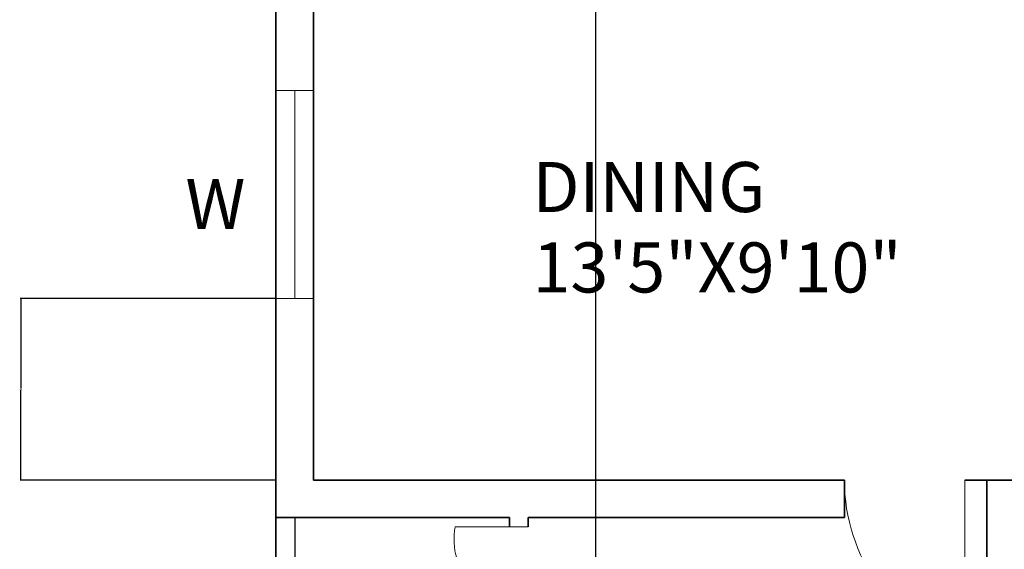
# Model space of a CAD drawing. Units: feet. Extents: x 5816 to 6644, y 25475 to 26788.
# Tile 5 of 23: x 5816 to 6052, y 26246 to 26373. Entities that reach past the tile are written whole.
import ezdxf

# ---------------------------------------------------------------- set-up
doc = ezdxf.new("R2010")
doc.units = ezdxf.units.FT
for name, color, linetype, lineweight in [('A-ANNO-DIMS', 2, 'Continuous', 13), ('A-ANNO-TEXT', 7, 'Continuous', 18), ('A-AREA-IDEN', 7, 'Continuous', 18), ('A-DOOR', 3, 'Continuous', 18), ('A-FLOR-RAIL', 8, 'Continuous', 25), ('A-GLAZ', 4, 'Continuous', 18), ('A-WALL', 7, 'Continuous', 35)]:
    doc.layers.add(name, color=color, linetype=linetype, lineweight=lineweight)
doc.styles.get("Standard").update_dxf_attribs({"font": 'arial.ttf'})
doc.dimstyles.get("Standard").update_dxf_attribs({"dimtxt": 0.18, "dimasz": 0.18, "dimexe": 0.18, "dimexo": 0.0625, "dimgap": 0.09, "dimtad": 0, "dimtih": 1, "dimtoh": 1, "dimdec": 4, "dimzin": 0, "dimdsep": 46, "dimtxsty": 'Standard', "dimcen": 0.09, "dimadec": 0, "dimazin": 0, "dimtfac": 1, "dimtdec": 4, "dimtofl": 0, "dimtmove": 0, "dimatfit": 3, "dimfxl": 1, "dimtolj": 1, "dimtzin": 0, "dimarcsym": 0})

# ---------------------------------------------------------------- blocks, each defined once
blk = doc.blocks.new('DOOR-KITCHEN')
blk.add_line((0, -40.87), (0, 0))
blk.add_arc((14.45, 0), 43.35, 180, 250.5286)
blk = doc.blocks.new('DOOR-SERVICE-BALCONY')
blk.add_line((-17.56, 0), (0, 0))
blk.add_arc((0, -2.91), 17.8, 170.5868, 270)
blk = doc.blocks.new('WIN-DINING')
for p, q in [((0, 0), (9, 0)), ((4.5, 0), (4.5, -49.84)), ((0, -49.84), (9, -49.84))]:
    blk.add_line(p, q)
blk = doc.blocks.new('*D58')
at = {"layer": 'A-ANNO-DIMS', "color": 0, "lineweight": -2, "transparency": 16777216}
for p, q in [((5953.98, 26168.65), (5953.98, 26787.91)), ((5954.16, 26787.73), (6030.2, 26787.73)), ((6106.8, 26787.73), (6030.76, 26787.73)), ((6106.98, 26168.71), (6106.98, 26787.91))]:
    blk.add_line(p, q, dxfattribs=at)
at = {"layer": 'A-ANNO-DIMS', "color": 0, "transparency": 16777216}
for points in [[(5954.16, 26787.76), (5954.16, 26787.7), (5953.98, 26787.73)], [(6106.8, 26787.76), (6106.8, 26787.7), (6106.98, 26787.73)]]:
    blk.add_solid(points, dxfattribs=at)
at = {"layer": 'Defpoints', "color": 0, "transparency": 16777216}
for p in [(6106.98, 26787.73), (5953.98, 26168.58), (6106.98, 26168.65)]:
    blk.add_point(p, dxfattribs=at)
at = {"layer": 'A-ANNO-DIMS', "color": 0, "transparency": 16777216, "insert": (6030.48, 26787.73), "char_height": 0.18, "attachment_point": 5}
blk.add_mtext('\\A1;153', dxfattribs=at)
blk = doc.blocks.new('*D66')
at = {"layer": 'A-ANNO-DIMS', "color": 0, "lineweight": -2, "transparency": 16777216}
for p, q in [((5877.25, 26306.14), (5815.98, 26306.14)), ((5816.16, 26305.96), (5816.16, 26284.54)), ((5816.16, 26262.76), (5816.16, 26284.18)), ((5877.25, 26262.58), (5815.98, 26262.58))]:
    blk.add_line(p, q, dxfattribs=at)
at = {"layer": 'A-ANNO-DIMS', "color": 0, "transparency": 16777216}
for points in [[(5816.13, 26305.96), (5816.19, 26305.96), (5816.16, 26306.14)], [(5816.13, 26262.76), (5816.19, 26262.76), (5816.16, 26262.58)]]:
    blk.add_solid(points, dxfattribs=at)
at = {"layer": 'Defpoints', "color": 0, "transparency": 16777216}
for p in [(5816.16, 26306.14), (5877.31, 26306.14), (5877.31, 26262.58)]:
    blk.add_point(p, dxfattribs=at)
at = {"layer": 'A-ANNO-DIMS', "color": 0, "transparency": 16777216, "insert": (5816.16, 26284.36), "char_height": 0.18, "attachment_point": 5}
blk.add_mtext('\\A1;43.55', dxfattribs=at)

msp = doc.modelspace()

# ---------------------------------------------------------------- linework, layer by layer
at = {"layer": 'A-FLOR-RAIL'}
msp.add_lwpolyline([(5881.8119, 26253.5846), (5881.8119, 26173.0846), (5933.3119, 26173.0846)], dxfattribs=at)
at = {"layer": 'A-WALL'}
for p, q in [((5877.3119, 26652.5846), (5877.3119, 26253.5846)), ((5877.3119, 26511.5846), (5877.3119, 26253.5846)), ((5877.3119, 26380.5846), (5877.3119, 26262.5846)), ((5886.3119, 26380.5846), (5886.3119, 26262.5846)), ((5877.3119, 26262.5846), (5877.3119, 26168.5846)), ((5886.3119, 26262.5846), (6013.6326, 26262.5846)), ((6013.6326, 26262.5846), (6013.6326, 26253.5846)), ((6042.532, 26262.5846), (6056.8119, 26262.5846)), ((6047.8119, 26177.5846), (6047.8119, 26262.5846)), ((5886.3119, 26253.5846), (5877.3119, 26253.5846)), ((5886.3119, 26253.5846), (5933.3119, 26253.5846)), ((5933.3119, 26253.5846), (5933.3119, 26251.4059)), ((5937.8119, 26253.5846), (5937.8119, 26251.4059)), ((5937.8119, 26253.5846), (6013.6326, 26253.5846))]:
    msp.add_line(p, q, dxfattribs=at)

# ---------------------------------------------------------------- block references
at = {"layer": 'A-DOOR'}
for name, p in [('DOOR-KITCHEN', (6042.532, 26262.5846)), ('DOOR-SERVICE-BALCONY', (5937.8119, 26251.4059))]:
    msp.add_blockref(name, p, dxfattribs=at)
at = {"layer": 'A-GLAZ'}
msp.add_blockref('WIN-DINING', (5877.3119, 26355.98), dxfattribs=at)

# ---------------------------------------------------------------- texts
at = {"layer": 'A-ANNO-DIMS'}
msp.add_text('13\'5"X9\'10"', height=12, dxfattribs=at).set_placement((5938.8522, 26307.5468))
at = {"layer": 'A-ANNO-TEXT'}
msp.add_text('W', height=12, dxfattribs=at).set_placement((5855.5998, 26322.7321))
at = {"layer": 'A-AREA-IDEN'}
msp.add_text('DINING', height=12, dxfattribs=at).set_placement((5938.8522, 26326.8237))

# ---------------------------------------------------------------- dimensions: what is measured, and where the dimension line sits
at = {"layer": 'A-ANNO-DIMS'}
dim = msp.add_linear_dim(base=(6106.9781, 26787.7346), p1=(5953.9781, 26168.5846), p2=(6106.9781, 26168.6509), dimstyle='Standard', override={"dimdec": 0, "dimlfac": 1, "dimrnd": 0, "dimzin": 0, "dimdsep": 46, "dimlunit": 2}, dxfattribs=at)
dim.commit()
dim.dimension.update_dxf_attribs({"geometry": '*D58', "text_midpoint": (6030.4781, 26787.7346)})
dim = msp.add_linear_dim(base=(5816.1619, 26306.1357), p1=(5877.3119, 26262.5846), p2=(5877.3119, 26306.1357), angle=90, dimstyle='Standard', override={"dimdec": 2, "dimlfac": 1, "dimrnd": 0, "dimzin": 0, "dimdsep": 46, "dimlunit": 2}, dxfattribs=at)
dim.commit()
dim.dimension.update_dxf_attribs({"geometry": '*D66', "text_midpoint": (5816.1619, 26284.3602)})

doc.saveas('drawing.dxf')
